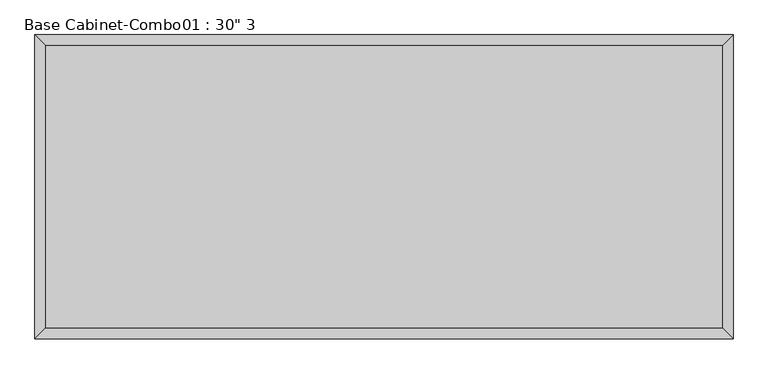
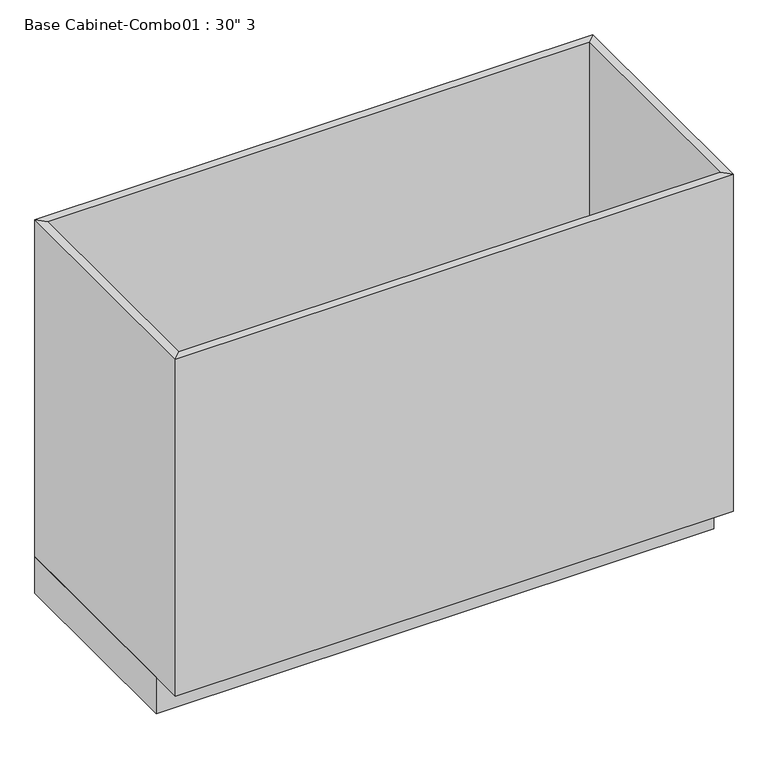
"""IFC4 building model written with IfcOpenShell, lengths in millimetres: furniture geometry."""

from ifc_helpers import new_model, si_unit, frame, origin, origin_with_axes, place, context, project, spatial, polyline, outline, extrude, faceted_brep, source, transform, mapped, element, save


def furniture_5f863b49(model_context):
    return source(origin(), model_context, "Body", "SolidModel", [
        extrude(outline(polyline([(660.0877049, 0.0), (660.0877049, -482.6), (-622.6122951, -482.6), (-622.6122951, 0.0), (660.0877049, 0.0)])), origin_with_axes(), (0.0, 0.0, 1.0), 88.9),
        faceted_brep([(641.0377049, -539.75, 908.05), (641.0377049, -539.75, 88.9), (-603.5622951, -539.75, 88.9), (-603.5622951, -539.75, 908.05), (660.0877049, -558.8, 908.05), (-622.6122951, -558.8, 908.05), (660.0877049, -558.8, 88.9), (-622.6122951, -558.8, 88.9), (-603.5622951, -19.05, 88.9), (-603.5622951, -19.05, 908.05), (-622.6122951, 0.0, 908.05), (-622.6122951, 0.0, 88.9), (641.0377049, -19.05, 88.9), (641.0377049, -19.05, 908.05), (660.0877049, 0.0, 908.05), (660.0877049, 0.0, 88.9)], [[[0, 1, 2, 3]], [[4, 0, 3, 5]], [[6, 4, 5, 7]], [[1, 6, 7, 2]], [[3, 2, 8, 9]], [[5, 3, 9, 10]], [[7, 5, 10, 11]], [[2, 7, 11, 8]], [[9, 8, 12, 13]], [[10, 9, 13, 14]], [[11, 10, 14, 15]], [[8, 11, 15, 12]], [[13, 12, 1, 0]], [[14, 13, 0, 4]], [[15, 14, 4, 6]], [[12, 15, 6, 1]]]),
        extrude(outline(polyline([(641.0377049, -19.05), (641.0377049, -539.75), (-603.5622951, -539.75), (-603.5622951, -19.05), (641.0377049, -19.05)])), frame((0.0, 0.0, 88.9), z_axis=(0.0, 0.0, 1.0), x_axis=(1.0, 0.0, 0.0)), (0.0, 0.0, 1.0), 19.05),
    ])


if __name__ == "__main__":
    model = new_model("IFC4")
    model_context = context("Model", 3, world=origin())
    ifc_project = project(units=[si_unit("LENGTHUNIT", "METRE", prefix="MILLI")], contexts=[model_context])
    site = spatial("IfcSite", under=ifc_project)
    building = spatial("IfcBuilding", under=site)
    placement = place(None, origin())
    furniture_shape = furniture_5f863b49(model_context)
    element("IfcFurniture", 1, ObjectType="Base Cabinet-Combo01 : 30\" 3", at=placement, inside=building, context=model_context, shape_type="MappedRepresentation", body=[
        mapped(furniture_shape, transform((0.0, 0.0, 0.0), x_axis=(1.0, 0.0, 0.0), y_axis=(0.0, 1.0, 0.0), z_axis=(0.0, 0.0, 1.0))),
    ])
    save(model, "model.ifc")

# Revit data of these elements
# Type "Base Cabinet-Combo01 : 30\" 3"
#   Depth = 1' - 10"
#   Height = 2' - 11 3/4"
#   Toe Depth = 0' - 3"
#   Toe Height = 0' - 3 1/2"
#   Width = 4' - 2 1/2"
#   Default Elevation = 0
# Element 1 (IfcFurniture, "Base Cabinet-Combo01 : 30\" 3")
#   Materials on its faces: "Cabinet"
# Materials
#   "Cabinet": colour RGB 204 122 2, transparency 0
